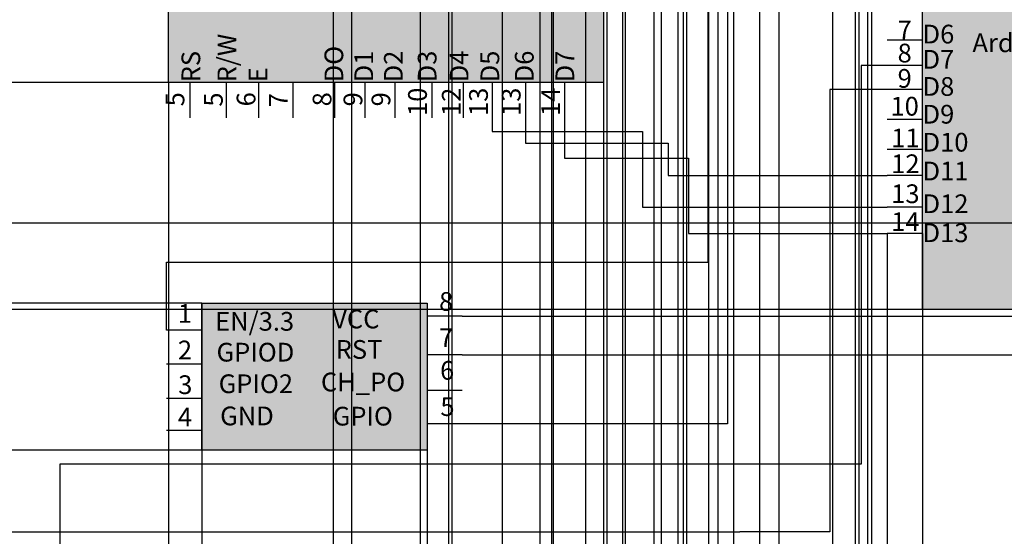
# Model space of a CAD drawing. Units: inches. Extents: x 35362 to 73946, y 43607 to 67532.
# Tile 128 of 134: x 46225 to 57838, y 50677 to 56772. Entities that reach past the tile are written whole.
import ezdxf

# ---------------------------------------------------------------- set-up
doc = ezdxf.new("R2010")
doc.units = ezdxf.units.IN
doc.header["$MEASUREMENT"] = 0
for name, color, linetype, lineweight in [('A-ANNO-DIMS', 2, 'Continuous', 18), ('E-ANNO-TEXT', 5, 'Continuous', 18), ('E-SYMB', 1, 'Continuous', 25), ('E-SYMB-PATT', 1, 'Continuous', 13), ('E-WIRE', 3, 'Continuous', 25)]:
    doc.layers.add(name, color=color, linetype=linetype, lineweight=lineweight)
doc.styles.get("Standard").update_dxf_attribs({"font": 'arial.ttf'})
doc.dimstyles.get("Standard").update_dxf_attribs({"dimtxt": 0.18, "dimasz": 0.18, "dimexe": 0.18, "dimexo": 0.0625, "dimgap": 0.09, "dimtad": 0, "dimtih": 1, "dimtoh": 1, "dimdec": 4, "dimzin": 0, "dimdsep": 46, "dimtxsty": 'Standard', "dimcen": 0.09, "dimadec": 0, "dimazin": 0, "dimtfac": 1, "dimtdec": 4, "dimtofl": 0, "dimtmove": 0, "dimatfit": 3, "dimfxl": 1, "dimtolj": 1, "dimtzin": 0, "dimarcsym": 0})

# ---------------------------------------------------------------- blocks, each defined once
blk = doc.blocks.new('*D11')
at = {"layer": 'A-ANNO-DIMS', "color": 0, "lineweight": -2, "transparency": 16777216}
for p, q in [((47979, 56029), (47979, 43607)), ((53110, 56029), (53110, 43607)), ((47979, 43607), (50544, 43607)), ((53110, 43607), (50545, 43607))]:
    blk.add_line(p, q, dxfattribs=at)
at = {"layer": 'A-ANNO-DIMS', "color": 0, "transparency": 16777216}
for points in [[(47979, 43607), (47979, 43607), (47979, 43607)], [(53110, 43607), (53110, 43607), (53110, 43607)]]:
    blk.add_solid(points, dxfattribs=at)
at = {"layer": 'Defpoints', "color": 0, "transparency": 16777216}
for p in [(47979, 56029), (53110, 56029), (53110, 43607)]:
    blk.add_point(p, dxfattribs=at)
at = {"layer": 'A-ANNO-DIMS', "color": 0, "transparency": 16777216, "insert": (50544, 43607), "char_height": 0.18, "attachment_point": 5}
blk.add_mtext('\\A1;5131', dxfattribs=at)
blk = doc.blocks.new('*D12')
at = {"layer": 'A-ANNO-DIMS', "color": 0, "lineweight": -2, "transparency": 16777216}
for p, q in [((47979, 59023), (35362, 59023)), ((35362, 59023), (35362, 57526)), ((35362, 56029), (35362, 57526)), ((47979, 56029), (35362, 56029))]:
    blk.add_line(p, q, dxfattribs=at)
at = {"layer": 'A-ANNO-DIMS', "color": 0, "transparency": 16777216}
for points in [[(35362, 59023), (35362, 59023), (35362, 59023)], [(35362, 56029), (35362, 56029), (35362, 56029)]]:
    blk.add_solid(points, dxfattribs=at)
at = {"layer": 'Defpoints', "color": 0, "transparency": 16777216}
for p in [(47979, 59023), (35362, 56029), (47979, 56029)]:
    blk.add_point(p, dxfattribs=at)
at = {"layer": 'A-ANNO-DIMS', "color": 0, "transparency": 16777216, "insert": (35362, 57526), "char_height": 0.18, "attachment_point": 5}
blk.add_mtext('\\A1;2994.4', dxfattribs=at)
blk = doc.blocks.new('*D13')
at = {"layer": 'A-ANNO-DIMS', "color": 0, "lineweight": -2, "transparency": 16777216}
for p, q in [((48373, 51694), (48373, 43607)), ((51029, 51694), (51029, 43607)), ((48374, 43607), (49701, 43607)), ((51029, 43607), (49702, 43607))]:
    blk.add_line(p, q, dxfattribs=at)
at = {"layer": 'A-ANNO-DIMS', "color": 0, "transparency": 16777216}
for points in [[(48374, 43607), (48374, 43607), (48373, 43607)], [(51029, 43607), (51029, 43607), (51029, 43607)]]:
    blk.add_solid(points, dxfattribs=at)
at = {"layer": 'Defpoints', "color": 0, "transparency": 16777216}
for p in [(48373, 51694), (51029, 51694), (51029, 43607)]:
    blk.add_point(p, dxfattribs=at)
at = {"layer": 'A-ANNO-DIMS', "color": 0, "transparency": 16777216, "insert": (49701, 43607), "char_height": 0.18, "attachment_point": 5}
blk.add_mtext('\\A1;2655.6', dxfattribs=at)
blk = doc.blocks.new('*D14')
at = {"layer": 'A-ANNO-DIMS', "color": 0, "lineweight": -2, "transparency": 16777216}
for p, q in [((48373, 53429), (35362, 53429)), ((35362, 53429), (35362, 52562)), ((35362, 51694), (35362, 52561)), ((48373, 51694), (35362, 51694))]:
    blk.add_line(p, q, dxfattribs=at)
at = {"layer": 'A-ANNO-DIMS', "color": 0, "transparency": 16777216}
for points in [[(35362, 53429), (35362, 53429), (35362, 53429)], [(35362, 51694), (35362, 51694), (35362, 51694)]]:
    blk.add_solid(points, dxfattribs=at)
at = {"layer": 'Defpoints', "color": 0, "transparency": 16777216}
for p in [(48373, 53429), (35362, 51694), (48373, 51694)]:
    blk.add_point(p, dxfattribs=at)
at = {"layer": 'A-ANNO-DIMS', "color": 0, "transparency": 16777216, "insert": (35362, 52562), "char_height": 0.18, "attachment_point": 5}
blk.add_mtext('\\A1;1735', dxfattribs=at)
blk = doc.blocks.new('*D17')
at = {"layer": 'A-ANNO-DIMS', "color": 0, "lineweight": -2, "transparency": 16777216}
for p, q in [((49923, 61293), (49923, 43607)), ((51914, 61293), (51914, 43607)), ((49923, 43607), (50918, 43607)), ((51914, 43607), (50919, 43607))]:
    blk.add_line(p, q, dxfattribs=at)
at = {"layer": 'A-ANNO-DIMS', "color": 0, "transparency": 16777216}
for points in [[(49923, 43607), (49923, 43607), (49923, 43607)], [(51914, 43607), (51914, 43607), (51914, 43607)]]:
    blk.add_solid(points, dxfattribs=at)
at = {"layer": 'Defpoints', "color": 0, "transparency": 16777216}
for p in [(49923, 61293), (51914, 61293), (51914, 43607)]:
    blk.add_point(p, dxfattribs=at)
at = {"layer": 'A-ANNO-DIMS', "color": 0, "transparency": 16777216, "insert": (50919, 43607), "char_height": 0.18, "attachment_point": 5}
blk.add_mtext('\\A1;1990.6', dxfattribs=at)
blk = doc.blocks.new('*D26')
at = {"layer": 'A-ANNO-DIMS', "color": 0, "lineweight": -2, "transparency": 16777216}
for p, q in [((47979, 56029), (35362, 56029)), ((35362, 56029), (35362, 54729)), ((35362, 53429), (35362, 54729)), ((48373, 53429), (35362, 53429))]:
    blk.add_line(p, q, dxfattribs=at)
at = {"layer": 'A-ANNO-DIMS', "color": 0, "transparency": 16777216}
for points in [[(35362, 56029), (35362, 56029), (35362, 56029)], [(35362, 53429), (35362, 53429), (35362, 53429)]]:
    blk.add_solid(points, dxfattribs=at)
at = {"layer": 'Defpoints', "color": 0, "transparency": 16777216}
for p in [(35362, 56029), (47979, 56029), (48373, 53429)]:
    blk.add_point(p, dxfattribs=at)
at = {"layer": 'A-ANNO-DIMS', "color": 0, "transparency": 16777216, "insert": (35362, 54729), "char_height": 0.18, "attachment_point": 5}
blk.add_mtext('\\A1;2599.8', dxfattribs=at)
blk = doc.blocks.new('*D27')
at = {"layer": 'A-ANNO-DIMS', "color": 0, "lineweight": -2, "transparency": 16777216}
for p, q in [((47979, 56029), (47979, 43607)), ((48373, 53429), (48373, 43607)), ((47979, 43607), (48176, 43607)), ((48373, 43607), (48176, 43607))]:
    blk.add_line(p, q, dxfattribs=at)
at = {"layer": 'A-ANNO-DIMS', "color": 0, "transparency": 16777216}
for points in [[(47979, 43607), (47979, 43607), (47979, 43607)], [(48373, 43607), (48373, 43607), (48373, 43607)]]:
    blk.add_solid(points, dxfattribs=at)
at = {"layer": 'Defpoints', "color": 0, "transparency": 16777216}
for p in [(47979, 56029), (48373, 53429), (48373, 43607)]:
    blk.add_point(p, dxfattribs=at)
at = {"layer": 'A-ANNO-DIMS', "color": 0, "transparency": 16777216, "insert": (48176, 43607), "char_height": 0.18, "attachment_point": 5}
blk.add_mtext('\\A1;394.8', dxfattribs=at)
blk = doc.blocks.new('*D36')
at = {"layer": 'A-ANNO-DIMS', "color": 0, "lineweight": -2, "transparency": 16777216}
for p, q in [((68321, 60122), (35362, 60122)), ((35362, 60122), (35362, 57248)), ((35362, 54373), (35362, 57247)), ((68321, 54373), (35362, 54373))]:
    blk.add_line(p, q, dxfattribs=at)
at = {"layer": 'A-ANNO-DIMS', "color": 0, "transparency": 16777216}
for points in [[(35362, 60122), (35362, 60122), (35362, 60122)], [(35362, 54373), (35362, 54373), (35362, 54373)]]:
    blk.add_solid(points, dxfattribs=at)
at = {"layer": 'Defpoints', "color": 0, "transparency": 16777216}
for p in [(68321, 60122), (35362, 54373), (68321, 54373)]:
    blk.add_point(p, dxfattribs=at)
at = {"layer": 'A-ANNO-DIMS', "color": 0, "transparency": 16777216, "insert": (35362, 57248), "char_height": 0.18, "attachment_point": 5}
blk.add_mtext('\\A1;5749.4', dxfattribs=at)
blk = doc.blocks.new('*D39')
at = {"layer": 'A-ANNO-DIMS', "color": 0, "lineweight": -2, "transparency": 16777216}
for p, q in [((53794, 46129), (53794, 67532)), ((53794, 67532), (54487, 67532)), ((55181, 67532), (54488, 67532)), ((55182, 46129), (55182, 67532))]:
    blk.add_line(p, q, dxfattribs=at)
at = {"layer": 'A-ANNO-DIMS', "color": 0, "transparency": 16777216}
for points in [[(53794, 67532), (53794, 67531), (53794, 67532)], [(55181, 67532), (55181, 67531), (55182, 67532)]]:
    blk.add_solid(points, dxfattribs=at)
at = {"layer": 'Defpoints', "color": 0, "transparency": 16777216}
for p in [(55182, 67532), (53794, 46129), (55182, 46129)]:
    blk.add_point(p, dxfattribs=at)
at = {"layer": 'A-ANNO-DIMS', "color": 0, "transparency": 16777216, "insert": (54488, 67532), "char_height": 0.18, "attachment_point": 5}
blk.add_mtext('\\A1;1388.0', dxfattribs=at)
blk = doc.blocks.new('*D40')
at = {"layer": 'A-ANNO-DIMS', "color": 0, "lineweight": -2, "transparency": 16777216}
for p, q in [((56874, 53352), (35362, 53352)), ((35362, 53351), (35362, 51333)), ((35362, 49315), (35362, 51333)), ((51806, 49315), (35362, 49315))]:
    blk.add_line(p, q, dxfattribs=at)
at = {"layer": 'A-ANNO-DIMS', "color": 0, "transparency": 16777216}
for points in [[(35362, 53351), (35362, 53351), (35362, 53352)], [(35362, 49315), (35362, 49315), (35362, 49315)]]:
    blk.add_solid(points, dxfattribs=at)
at = {"layer": 'Defpoints', "color": 0, "transparency": 16777216}
for p in [(35362, 53352), (56874, 53352), (51807, 49315)]:
    blk.add_point(p, dxfattribs=at)
at = {"layer": 'A-ANNO-DIMS', "color": 0, "transparency": 16777216, "insert": (35362, 51333), "char_height": 0.18, "attachment_point": 5}
blk.add_mtext('\\A1;4036.9', dxfattribs=at)
blk = doc.blocks.new('*D44')
at = {"layer": 'A-ANNO-DIMS', "color": 0, "lineweight": -2, "transparency": 16777216}
for p, q in [((52518, 64828), (52518, 43607)), ((54091, 64828), (54091, 43607)), ((52518, 43607), (53304, 43607)), ((54091, 43607), (53305, 43607))]:
    blk.add_line(p, q, dxfattribs=at)
at = {"layer": 'A-ANNO-DIMS', "color": 0, "transparency": 16777216}
for points in [[(52518, 43607), (52518, 43607), (52518, 43607)], [(54091, 43607), (54091, 43607), (54091, 43607)]]:
    blk.add_solid(points, dxfattribs=at)
at = {"layer": 'Defpoints', "color": 0, "transparency": 16777216}
for p in [(52518, 64829), (54091, 64829), (54091, 43607)]:
    blk.add_point(p, dxfattribs=at)
at = {"layer": 'A-ANNO-DIMS', "color": 0, "transparency": 16777216, "insert": (53304, 43607), "char_height": 0.18, "attachment_point": 5}
blk.add_mtext('\\A1;1573.0', dxfattribs=at)
blk = doc.blocks.new('*D49')
at = {"layer": 'A-ANNO-DIMS', "color": 0, "lineweight": -2, "transparency": 16777216}
for p, q in [((56457, 54250), (56457, 43607)), ((56874, 54250), (56874, 43607)), ((56457, 43607), (56665, 43607)), ((56873, 43607), (56666, 43607))]:
    blk.add_line(p, q, dxfattribs=at)
at = {"layer": 'A-ANNO-DIMS', "color": 0, "transparency": 16777216}
for points in [[(56457, 43607), (56457, 43607), (56457, 43607)], [(56873, 43607), (56873, 43607), (56874, 43607)]]:
    blk.add_solid(points, dxfattribs=at)
at = {"layer": 'Defpoints', "color": 0, "transparency": 16777216}
for p in [(56457, 54250), (56874, 54250), (56874, 43607)]:
    blk.add_point(p, dxfattribs=at)
at = {"layer": 'A-ANNO-DIMS', "color": 0, "transparency": 16777216, "insert": (56665, 43607), "char_height": 0.18, "attachment_point": 5}
blk.add_mtext('\\A1;416.3', dxfattribs=at)
blk = doc.blocks.new('*D53')
at = {"layer": 'A-ANNO-DIMS', "color": 0, "lineweight": -2, "transparency": 16777216}
for p, q in [((56874, 53351), (56874, 43607)), ((58225, 52935), (58225, 43607)), ((56874, 43607), (57549, 43607)), ((58225, 43607), (57550, 43607))]:
    blk.add_line(p, q, dxfattribs=at)
at = {"layer": 'A-ANNO-DIMS', "color": 0, "transparency": 16777216}
for points in [[(56874, 43607), (56874, 43607), (56874, 43607)], [(58225, 43607), (58225, 43607), (58225, 43607)]]:
    blk.add_solid(points, dxfattribs=at)
at = {"layer": 'Defpoints', "color": 0, "transparency": 16777216}
for p in [(56874, 53352), (58225, 52935), (58225, 43607)]:
    blk.add_point(p, dxfattribs=at)
at = {"layer": 'A-ANNO-DIMS', "color": 0, "transparency": 16777216, "insert": (57549, 43607), "char_height": 0.18, "attachment_point": 5}
blk.add_mtext('\\A1;1351.2', dxfattribs=at)
blk = doc.blocks.new('*D57')
at = {"layer": 'A-ANNO-DIMS', "color": 0, "lineweight": -2, "transparency": 16777216}
for p, q in [((51445, 53273), (73946, 53273)), ((73946, 53273), (73946, 53046)), ((73946, 52819), (73946, 53045)), ((51445, 52819), (73946, 52819))]:
    blk.add_line(p, q, dxfattribs=at)
at = {"layer": 'A-ANNO-DIMS', "color": 0, "transparency": 16777216}
for points in [[(73946, 53273), (73946, 53273), (73946, 53273)], [(73946, 52819), (73946, 52819), (73946, 52819)]]:
    blk.add_solid(points, dxfattribs=at)
at = {"layer": 'Defpoints', "color": 0, "transparency": 16777216}
for p in [(51445, 53273), (51445, 52819), (73946, 52819)]:
    blk.add_point(p, dxfattribs=at)
at = {"layer": 'A-ANNO-DIMS', "color": 0, "transparency": 16777216, "insert": (73946, 53046), "char_height": 0.18, "attachment_point": 5}
blk.add_mtext('\\A1;454.2', dxfattribs=at)
blk = doc.blocks.new('*D67')
at = {"layer": 'A-ANNO-DIMS', "color": 0, "lineweight": -2, "transparency": 16777216}
for p, q in [((56874, 53352), (35362, 53352)), ((35362, 53351), (35362, 49401)), ((35362, 45450), (35362, 49401)), ((53794, 45450), (35362, 45450))]:
    blk.add_line(p, q, dxfattribs=at)
at = {"layer": 'A-ANNO-DIMS', "color": 0, "transparency": 16777216}
for points in [[(35362, 53351), (35362, 53351), (35362, 53352)], [(35362, 45450), (35362, 45450), (35362, 45450)]]:
    blk.add_solid(points, dxfattribs=at)
at = {"layer": 'Defpoints', "color": 0, "transparency": 16777216}
for p in [(35362, 53352), (56874, 53352), (53794, 45450)]:
    blk.add_point(p, dxfattribs=at)
at = {"layer": 'A-ANNO-DIMS', "color": 0, "transparency": 16777216, "insert": (35362, 49401), "char_height": 0.18, "attachment_point": 5}
blk.add_mtext('\\A1;7901.6', dxfattribs=at)
blk = doc.blocks.new('*D77')
at = {"layer": 'A-ANNO-DIMS', "color": 0, "lineweight": -2, "transparency": 16777216}
for p, q in [((53794, 46129), (53794, 67532)), ((53794, 67532), (53923, 67532)), ((54053, 67532), (53924, 67532)), ((54053, 46555), (54053, 67532))]:
    blk.add_line(p, q, dxfattribs=at)
at = {"layer": 'A-ANNO-DIMS', "color": 0, "transparency": 16777216}
for points in [[(53794, 67532), (53794, 67531), (53794, 67532)], [(54053, 67532), (54053, 67531), (54053, 67532)]]:
    blk.add_solid(points, dxfattribs=at)
at = {"layer": 'Defpoints', "color": 0, "transparency": 16777216}
for p in [(54053, 67532), (54053, 46555), (53794, 46129)]:
    blk.add_point(p, dxfattribs=at)
at = {"layer": 'A-ANNO-DIMS', "color": 0, "transparency": 16777216, "insert": (53923, 67532), "char_height": 0.18, "attachment_point": 5}
blk.add_mtext('\\A1;259.26', dxfattribs=at)
blk = doc.blocks.new('*D78')
at = {"layer": 'A-ANNO-DIMS', "color": 0, "lineweight": -2, "transparency": 16777216}
for p, q in [((54053, 46555), (54053, 67532)), ((54053, 67532), (54203, 67532)), ((54353, 67532), (54203, 67532)), ((54353, 46555), (54353, 67532))]:
    blk.add_line(p, q, dxfattribs=at)
at = {"layer": 'A-ANNO-DIMS', "color": 0, "transparency": 16777216}
for points in [[(54053, 67532), (54053, 67531), (54053, 67532)], [(54353, 67532), (54353, 67531), (54353, 67532)]]:
    blk.add_solid(points, dxfattribs=at)
at = {"layer": 'Defpoints', "color": 0, "transparency": 16777216}
for p in [(54353, 67532), (54053, 46555), (54353, 46555)]:
    blk.add_point(p, dxfattribs=at)
at = {"layer": 'A-ANNO-DIMS', "color": 0, "transparency": 16777216, "insert": (54203, 67532), "char_height": 0.18, "attachment_point": 5}
blk.add_mtext('\\A1;300.2', dxfattribs=at)
blk = doc.blocks.new('*D79')
at = {"layer": 'A-ANNO-DIMS', "color": 0, "lineweight": -2, "transparency": 16777216}
for p, q in [((54353, 46555), (54353, 67532)), ((54353, 67532), (54500, 67532)), ((54648, 67532), (54501, 67532)), ((54648, 46555), (54648, 67532))]:
    blk.add_line(p, q, dxfattribs=at)
at = {"layer": 'A-ANNO-DIMS', "color": 0, "transparency": 16777216}
for points in [[(54353, 67532), (54353, 67531), (54353, 67532)], [(54648, 67532), (54648, 67531), (54648, 67532)]]:
    blk.add_solid(points, dxfattribs=at)
at = {"layer": 'Defpoints', "color": 0, "transparency": 16777216}
for p in [(54648, 67532), (54353, 46555), (54648, 46555)]:
    blk.add_point(p, dxfattribs=at)
at = {"layer": 'A-ANNO-DIMS', "color": 0, "transparency": 16777216, "insert": (54501, 67532), "char_height": 0.18, "attachment_point": 5}
blk.add_mtext('\\A1;295.1', dxfattribs=at)
blk = doc.blocks.new('*D80')
at = {"layer": 'A-ANNO-DIMS', "color": 0, "lineweight": -2, "transparency": 16777216}
for p, q in [((54648, 46555), (54648, 67532)), ((54648, 67532), (54800, 67532)), ((54953, 67532), (54801, 67532)), ((54953, 46555), (54953, 67532))]:
    blk.add_line(p, q, dxfattribs=at)
at = {"layer": 'A-ANNO-DIMS', "color": 0, "transparency": 16777216}
for points in [[(54648, 67532), (54648, 67531), (54648, 67532)], [(54953, 67532), (54953, 67531), (54953, 67532)]]:
    blk.add_solid(points, dxfattribs=at)
at = {"layer": 'Defpoints', "color": 0, "transparency": 16777216}
for p in [(54953, 67532), (54648, 46555), (54953, 46555)]:
    blk.add_point(p, dxfattribs=at)
at = {"layer": 'A-ANNO-DIMS', "color": 0, "transparency": 16777216, "insert": (54801, 67532), "char_height": 0.18, "attachment_point": 5}
blk.add_mtext('\\A1;305.27', dxfattribs=at)
blk = doc.blocks.new('*D82')
at = {"layer": 'A-ANNO-DIMS', "color": 0, "lineweight": -2, "transparency": 16777216}
for p, q in [((54464, 49315), (54464, 67532)), ((54465, 67532), (55139, 67532)), ((55815, 67532), (55140, 67532)), ((55815, 49110), (55815, 67532))]:
    blk.add_line(p, q, dxfattribs=at)
at = {"layer": 'A-ANNO-DIMS', "color": 0, "transparency": 16777216}
for points in [[(54465, 67532), (54465, 67531), (54464, 67532)], [(55815, 67532), (55815, 67531), (55815, 67532)]]:
    blk.add_solid(points, dxfattribs=at)
at = {"layer": 'Defpoints', "color": 0, "transparency": 16777216}
for p in [(55815, 67532), (54464, 49315), (55815, 49110)]:
    blk.add_point(p, dxfattribs=at)
at = {"layer": 'A-ANNO-DIMS', "color": 0, "transparency": 16777216, "insert": (55140, 67532), "char_height": 0.18, "attachment_point": 5}
blk.add_mtext('\\A1;1350.9', dxfattribs=at)
blk = doc.blocks.new('*D85')
at = {"layer": 'A-ANNO-DIMS', "color": 0, "lineweight": -2, "transparency": 16777216}
for p, q in [((50953, 49098), (50953, 67532)), ((50953, 67532), (51119, 67532)), ((51285, 67532), (51120, 67532)), ((51286, 49320), (51286, 67532))]:
    blk.add_line(p, q, dxfattribs=at)
at = {"layer": 'A-ANNO-DIMS', "color": 0, "transparency": 16777216}
for points in [[(50953, 67532), (50953, 67531), (50953, 67532)], [(51285, 67532), (51285, 67531), (51286, 67532)]]:
    blk.add_solid(points, dxfattribs=at)
at = {"layer": 'Defpoints', "color": 0, "transparency": 16777216}
for p in [(51286, 67532), (51286, 49320), (50953, 49098)]:
    blk.add_point(p, dxfattribs=at)
at = {"layer": 'A-ANNO-DIMS', "color": 0, "transparency": 16777216, "insert": (51119, 67532), "char_height": 0.18, "attachment_point": 5}
blk.add_mtext('\\A1;332.9', dxfattribs=at)
blk = doc.blocks.new('*D88')
at = {"layer": 'A-ANNO-DIMS', "color": 0, "lineweight": -2, "transparency": 16777216}
for p, q in [((52363, 48318), (52363, 67532)), ((52363, 67532), (52432, 67532)), ((52502, 67532), (52433, 67532)), ((52502, 48318), (52502, 67532))]:
    blk.add_line(p, q, dxfattribs=at)
at = {"layer": 'A-ANNO-DIMS', "color": 0, "transparency": 16777216}
for points in [[(52363, 67532), (52363, 67531), (52363, 67532)], [(52502, 67532), (52502, 67531), (52502, 67532)]]:
    blk.add_solid(points, dxfattribs=at)
at = {"layer": 'Defpoints', "color": 0, "transparency": 16777216}
for p in [(52502, 67532), (52363, 48318), (52502, 48318)]:
    blk.add_point(p, dxfattribs=at)
at = {"layer": 'A-ANNO-DIMS', "color": 0, "transparency": 16777216, "insert": (52432, 67532), "char_height": 0.18, "attachment_point": 5}
blk.add_mtext('\\A1;139.8', dxfattribs=at)
blk = doc.blocks.new('*D96')
at = {"layer": 'A-ANNO-DIMS', "color": 0, "lineweight": -2, "transparency": 16777216}
for p, q in [((53367, 64998), (53367, 43607)), ((53989, 64998), (53989, 43607)), ((53367, 43607), (53677, 43607)), ((53988, 43607), (53678, 43607))]:
    blk.add_line(p, q, dxfattribs=at)
at = {"layer": 'A-ANNO-DIMS', "color": 0, "transparency": 16777216}
for points in [[(53367, 43607), (53367, 43607), (53367, 43607)], [(53988, 43607), (53988, 43607), (53989, 43607)]]:
    blk.add_solid(points, dxfattribs=at)
at = {"layer": 'Defpoints', "color": 0, "transparency": 16777216}
for p in [(53367, 64998), (53989, 64998), (53989, 43607)]:
    blk.add_point(p, dxfattribs=at)
at = {"layer": 'A-ANNO-DIMS', "color": 0, "transparency": 16777216, "insert": (53678, 43607), "char_height": 0.18, "attachment_point": 5}
blk.add_mtext('\\A1;621.8', dxfattribs=at)
blk = doc.blocks.new('*D99')
at = {"layer": 'A-ANNO-DIMS', "color": 0, "lineweight": -2, "transparency": 16777216}
for p, q in [((52897, 65292), (52897, 43607)), ((52518, 64828), (52518, 43607)), ((52518, 43607), (52707, 43607)), ((52897, 43607), (52708, 43607))]:
    blk.add_line(p, q, dxfattribs=at)
at = {"layer": 'A-ANNO-DIMS', "color": 0, "transparency": 16777216}
for points in [[(52518, 43607), (52518, 43607), (52518, 43607)], [(52897, 43607), (52897, 43607), (52897, 43607)]]:
    blk.add_solid(points, dxfattribs=at)
at = {"layer": 'Defpoints', "color": 0, "transparency": 16777216}
for p in [(52897, 65292), (52518, 64829), (52897, 43607)]:
    blk.add_point(p, dxfattribs=at)
at = {"layer": 'A-ANNO-DIMS', "color": 0, "transparency": 16777216, "insert": (52708, 43607), "char_height": 0.18, "attachment_point": 5}
blk.add_mtext('\\A1;379.7', dxfattribs=at)
blk = doc.blocks.new('*D100')
at = {"layer": 'A-ANNO-DIMS', "color": 0, "lineweight": -2, "transparency": 16777216}
for p, q in [((52897, 65292), (52897, 43607)), ((53151, 64926), (53151, 43607)), ((52898, 43607), (53024, 43607)), ((53150, 43607), (53024, 43607))]:
    blk.add_line(p, q, dxfattribs=at)
at = {"layer": 'A-ANNO-DIMS', "color": 0, "transparency": 16777216}
for points in [[(52898, 43607), (52898, 43607), (52897, 43607)], [(53150, 43607), (53150, 43607), (53151, 43607)]]:
    blk.add_solid(points, dxfattribs=at)
at = {"layer": 'Defpoints', "color": 0, "transparency": 16777216}
for p in [(52897, 65292), (53151, 64926), (53151, 43607)]:
    blk.add_point(p, dxfattribs=at)
at = {"layer": 'A-ANNO-DIMS', "color": 0, "transparency": 16777216, "insert": (53024, 43607), "char_height": 0.18, "attachment_point": 5}
blk.add_mtext('\\A1;253.2', dxfattribs=at)
blk = doc.blocks.new('*D102')
at = {"layer": 'A-ANNO-DIMS', "color": 0, "lineweight": -2, "transparency": 16777216}
for p, q in [((56080, 63695), (56080, 43607)), ((56272, 63697), (56272, 43607)), ((56081, 43607), (56176, 43607)), ((56272, 43607), (56177, 43607))]:
    blk.add_line(p, q, dxfattribs=at)
at = {"layer": 'A-ANNO-DIMS', "color": 0, "transparency": 16777216}
for points in [[(56081, 43607), (56081, 43607), (56080, 43607)], [(56272, 43607), (56272, 43607), (56272, 43607)]]:
    blk.add_solid(points, dxfattribs=at)
at = {"layer": 'Defpoints', "color": 0, "transparency": 16777216}
for p in [(56080, 63695), (56272, 63697), (56272, 43607)]:
    blk.add_point(p, dxfattribs=at)
at = {"layer": 'A-ANNO-DIMS', "color": 0, "transparency": 16777216, "insert": (56176, 43607), "char_height": 0.18, "attachment_point": 5}
blk.add_mtext('\\A1;191.98', dxfattribs=at)
blk = doc.blocks.new('*D104')
at = {"layer": 'A-ANNO-DIMS', "color": 0, "lineweight": -2, "transparency": 16777216}
for p, q in [((56123, 63318), (56123, 43607)), ((56223, 63318), (56223, 43607)), ((56123, 43607), (56173, 43607)), ((56223, 43607), (56173, 43607))]:
    blk.add_line(p, q, dxfattribs=at)
at = {"layer": 'A-ANNO-DIMS', "color": 0, "transparency": 16777216}
for points in [[(56123, 43607), (56123, 43607), (56123, 43607)], [(56223, 43607), (56223, 43607), (56223, 43607)]]:
    blk.add_solid(points, dxfattribs=at)
at = {"layer": 'Defpoints', "color": 0, "transparency": 16777216}
for p in [(56123, 63318), (56223, 63318), (56223, 43607)]:
    blk.add_point(p, dxfattribs=at)
at = {"layer": 'A-ANNO-DIMS', "color": 0, "transparency": 16777216, "insert": (56173, 43607), "char_height": 0.18, "attachment_point": 5}
blk.add_mtext('\\A1;99.74', dxfattribs=at)
blk = doc.blocks.new('*D107')
at = {"layer": 'A-ANNO-DIMS', "color": 0, "lineweight": -2, "transparency": 16777216}
for p, q in [((50140, 59850), (50140, 43607)), ((51321, 59850), (51321, 43607)), ((50140, 43607), (50730, 43607)), ((51321, 43607), (50731, 43607))]:
    blk.add_line(p, q, dxfattribs=at)
at = {"layer": 'A-ANNO-DIMS', "color": 0, "transparency": 16777216}
for points in [[(50140, 43607), (50140, 43607), (50140, 43607)], [(51321, 43607), (51321, 43607), (51321, 43607)]]:
    blk.add_solid(points, dxfattribs=at)
at = {"layer": 'Defpoints', "color": 0, "transparency": 16777216}
for p in [(50140, 59850), (51321, 59850), (51321, 43607)]:
    blk.add_point(p, dxfattribs=at)
at = {"layer": 'A-ANNO-DIMS', "color": 0, "transparency": 16777216, "insert": (50730, 43607), "char_height": 0.18, "attachment_point": 5}
blk.add_mtext('\\A1;1181.3', dxfattribs=at)
blk = doc.blocks.new('*D112')
at = {"layer": 'A-ANNO-DIMS', "color": 0, "lineweight": -2, "transparency": 16777216}
for p, q in [((53333, 60113), (53333, 43607)), ((53705, 60126), (53705, 43607)), ((53333, 43607), (53519, 43607)), ((53705, 43607), (53519, 43607))]:
    blk.add_line(p, q, dxfattribs=at)
at = {"layer": 'A-ANNO-DIMS', "color": 0, "transparency": 16777216}
for points in [[(53333, 43607), (53333, 43607), (53333, 43607)], [(53705, 43607), (53705, 43607), (53705, 43607)]]:
    blk.add_solid(points, dxfattribs=at)
at = {"layer": 'Defpoints', "color": 0, "transparency": 16777216}
for p in [(53333, 60113), (53705, 60126), (53705, 43607)]:
    blk.add_point(p, dxfattribs=at)
at = {"layer": 'A-ANNO-DIMS', "color": 0, "transparency": 16777216, "insert": (53519, 43607), "char_height": 0.18, "attachment_point": 5}
blk.add_mtext('\\A1;372.6', dxfattribs=at)

msp = doc.modelspace()

# ---------------------------------------------------------------- hatches: boundary and pattern name
at = {"layer": 'E-SYMB-PATT'}
h = msp.add_hatch(color=256, dxfattribs=at)
h.dxf.hatch_style = 1
h.paths.add_polyline_path([(56873.602, 59185.144), (56873.602, 53351.529), (61240.907, 53351.529), (61240.907, 59185.144)])
h = msp.add_hatch(color=256, dxfattribs=at)
h.dxf.hatch_style = 1
h.paths.add_polyline_path([(53109.76, 56028.836), (53109.76, 59023.276), (47978.665, 59023.276), (47978.665, 56028.836)])
h = msp.add_hatch(color=256, dxfattribs=at)
h.dxf.hatch_style = 1
h.paths.add_polyline_path([(51029.043, 51694.087), (51029.043, 53429.019), (48373.492, 53429.019), (48373.492, 51694.087)])

# ---------------------------------------------------------------- linework, layer by layer
at = {"layer": 'E-SYMB'}
for p, q in [((56873.602, 56528.919), (56457.29, 56528.919)), ((56873.602, 56231.74), (56457.29, 56231.74)), ((48230.625, 56028.836), (48230.625, 55612.524)), ((48660.098, 56028.836), (48660.098, 55612.524)), ((49041.599, 56028.836), (49041.599, 55612.524)), ((49447.981, 56028.836), (49447.981, 55612.524)), ((49937.463, 56028.836), (49937.463, 55612.524)), ((50296.119, 56028.836), (50296.119, 55612.524)), ((50650.395, 56028.836), (50650.395, 55612.524)), ((51087.024, 56028.836), (51087.024, 55612.524)), ((51455.229, 56028.836), (51455.229, 55612.524)), ((51797.894, 56028.836), (51797.894, 55612.524)), ((52188.791, 56028.836), (52188.791, 55612.524)), ((52650.246, 56028.836), (52650.246, 55612.524)), ((56873.602, 55948.948), (56457.29, 55948.948)), ((56873.602, 55593.178), (56457.29, 55593.178)), ((56873.602, 55241.1), (56457.29, 55241.1)), ((56873.602, 54934.69), (56457.29, 54934.69)), ((56873.602, 54560.675), (56457.29, 54560.675)), ((56873.602, 54249.826), (56457.29, 54249.826)), ((51445.356, 53272.782), (51029.043, 53272.782)), ((48373.492, 53109.735), (47957.179, 53109.735)), ((51445.356, 52818.57), (51029.043, 52818.57)), ((48373.492, 52706.392), (47957.179, 52706.392)), ((51445.356, 52397.789), (51029.043, 52397.789)), ((48373.492, 52303.049), (47957.179, 52303.049)), ((48373.492, 51923.785), (47957.179, 51923.785)), ((51445.356, 52004.266), (51029.043, 52004.266))]:
    msp.add_line(p, q, dxfattribs=at)
for points in [[(56873.602, 59185.144), (61240.907, 59185.144), (61240.907, 53351.529), (56873.602, 53351.529)], [(47978.665, 59023.276), (53109.76, 59023.276), (53109.76, 56028.836), (47978.665, 56028.836)], [(48373.492, 53429.019), (51029.043, 53429.019), (51029.043, 51694.087), (48373.492, 51694.087)]]:
    msp.add_lwpolyline(points, close=True, dxfattribs=at)
at = {"layer": 'E-WIRE'}
for p, q in [((54572.84, 58474.868), (54572.84, 52004.266)), ((54344.773, 53911.892), (54344.773, 58146.959)), ((56457.29, 56231.74), (56150.086, 56231.74)), ((56150.086, 56231.74), (56150.086, 53577.957)), ((56457.29, 55948.948), (55781.317, 55948.948)), ((55781.317, 55948.948), (55781.317, 53662.393)), ((51797.894, 55612.524), (51797.894, 55453.525)), ((52188.791, 55612.524), (52188.791, 55313.853)), ((52650.246, 55612.524), (52650.246, 55136.134)), ((51797.894, 55453.525), (53572.548, 55453.525)), ((53572.548, 55453.525), (53572.548, 54560.675)), ((52188.791, 55313.853), (53871.419, 55313.853)), ((53871.419, 55313.853), (53871.419, 54934.69)), ((52650.246, 55136.134), (54114.113, 55136.134)), ((54114.113, 55136.134), (54114.113, 54249.826)), ((53871.419, 54934.69), (56457.29, 54934.69)), ((53572.548, 54560.675), (56457.29, 54560.675)), ((54114.113, 54249.826), (56457.29, 54249.826)), ((47957.179, 53109.735), (47957.179, 53911.892)), ((47957.179, 53911.892), (54344.773, 53911.892)), ((55781.317, 53662.393), (55781.317, 50729.557)), ((56150.086, 53577.957), (56150.086, 51529.852)), ((54572.84, 52004.266), (51445.356, 52004.266)), ((56150.086, 51529.852), (46698.777, 51529.852)), ((46698.777, 51529.852), (46698.777, 49689.843)), ((38575.774, 50731.821), (54718.752, 50731.821)), ((55781.317, 50729.557), (54718.752, 50731.821))]:
    msp.add_line(p, q, dxfattribs=at)

# ---------------------------------------------------------------- texts
at = {"layer": 'E-ANNO-TEXT'}
for s, height, p in [('7', 220.866, (56579.272, 56539.848)), ('D6', 220.866, (56873.602, 56491.012)), ('Arduino_UNO_R3', 220.86598, (57462.175, 56388.42)), ('8', 220.866, (56579.272, 56267.244)), ('D7', 220.866, (56873.602, 56193.637)), ('9', 220.866, (56579.272, 55968.56)), ('D8', 220.866, (56873.602, 55873.308)), ('10', 220.866, (56495.329, 55640.201)), ('D9', 220.866, (56873.602, 55545.826)), ('11', 220.866, (56504.349, 55265.371)), ('D10', 220.866, (56873.602, 55215.796)), ('12', 220.866, (56504.349, 54961.475)), ('D11', 220.866, (56873.602, 54875.374)), ('13', 220.866, (56504.349, 54607.867)), ('D12', 220.866, (56873.602, 54489.594)), ('14', 220.866, (56504.349, 54277.862)), ('D13', 220.866, (56873.602, 54147.25)), ('8', 220.866, (51171.439, 53337.11)), ('1', 220.866, (48090.611, 53195.947)), ('EN/3.3', 220.866, (48529.899, 53102.666)), ('VCC', 220.866, (49910.79, 53130.109)), ('7', 220.866, (51171.439, 52909.545)), ('2', 220.866, (48090.611, 52764.53)), ('GPIOD', 220.866, (48546.394, 52738.909)), ('RST', 220.866, (49951.348, 52771.119)), ('6', 220.866, (51183.005, 52524.352)), ('CH_PO', 220.866, (49777.527, 52386.999)), ('3', 220.866, (48094.256, 52355.135)), ('GPIO2', 220.866, (48571.252, 52366.37)), ('5', 220.866, (51186.86, 52096.787)), ('4', 220.866, (48090.401, 51973.794)), ('GND', 220.866, (48589.007, 51986.734)), ('GPIO', 220.866, (49916.584, 51983.869))]:
    msp.add_text(s, height=height, dxfattribs=at).set_placement(p)
for s, p in [('R/W', (48779.04, 56031.884)), ('DO', (50040.812, 56031.884)), ('RS ', (48353.855, 56031.884)), ('D1', (50393.227, 56031.884)), ('D2', (50742.633, 56031.884)), ('D3', (51141.004, 56031.884)), ('D4', (51518.064, 56031.884)), ('D5', (51880.508, 56031.884)), ('D6', (52286.763, 56031.884)), ('D7', (52765.285, 56031.884)), ('E ', (49144.507, 56031.884)), ('5', (48166.52, 55748.862)), ('5', (48619.301, 55745.805)), ('6', (49004.776, 55748.862)), ('7', (49386.164, 55738.929)), ('8', (49901.16, 55748.862)), ('9', (50265.572, 55748.862)), ('9', (50595.98, 55748.862)), ('10', (51027.192, 55635.623)), ('12', (51425.475, 55635.623)), ('13', (51746.704, 55635.623)), ('13', (52132.18, 55635.623)), ('14', (52597.198, 55635.623))]:
    msp.add_text(s, height=220.866, rotation=90, dxfattribs=at).set_placement(p)

# ---------------------------------------------------------------- dimensions: what is measured, and where the dimension line sits
at = {"layer": 'A-ANNO-DIMS'}
for base, p1, p2, override, picture, middle in [((51285.595, 67531.512), (50952.662, 49098.368), (51285.595, 49320.079), {"dimdec": 1, "dimlfac": 1, "dimrnd": 0, "dimzin": 0, "dimdsep": 46, "dimlunit": 2}, '*D85', (51119.128, 67531.512)), ((52502.363, 67531.512), (52362.557, 48318.269), (52502.363, 48318.269), {"dimdec": 1, "dimlfac": 1, "dimrnd": 0, "dimzin": 0, "dimdsep": 46, "dimlunit": 2}, '*D88', (52432.46, 67531.512)), ((55181.634, 67531.512), (53793.638, 46128.878), (55181.634, 46128.878), {"dimdec": 1, "dimlfac": 1, "dimrnd": 0, "dimzin": 0, "dimdsep": 46, "dimlunit": 2}, '*D39', (54487.636, 67531.512)), ((54052.899, 67531.512), (53793.638, 46128.878), (54052.899, 46555.293), {"dimdec": 2, "dimlfac": 1, "dimrnd": 0, "dimzin": 0, "dimdsep": 46, "dimlunit": 2}, '*D77', (53923.269, 67531.512)), ((54353.08, 67531.512), (54052.899, 46555.293), (54353.08, 46555.293), {"dimdec": 1, "dimlfac": 1, "dimrnd": 0, "dimzin": 0, "dimdsep": 46, "dimlunit": 2}, '*D78', (54202.99, 67531.512)), ((54648.173, 67531.512), (54353.08, 46555.293), (54648.173, 46555.293), {"dimdec": 1, "dimlfac": 1, "dimrnd": 0, "dimzin": 0, "dimdsep": 46, "dimlunit": 2}, '*D79', (54500.627, 67531.512)), ((55815.319, 67531.512), (54464.399, 49314.669), (55815.319, 49110.104), {"dimdec": 1, "dimlfac": 1, "dimrnd": 0, "dimzin": 0, "dimdsep": 46, "dimlunit": 2}, '*D82', (55139.859, 67531.512)), ((54953.441, 67531.512), (54648.173, 46555.293), (54953.441, 46555.293), {"dimdec": 2, "dimlfac": 1, "dimrnd": 0, "dimzin": 0, "dimdsep": 46, "dimlunit": 2}, '*D80', (54800.807, 67531.512)), ((52897.48, 43606.859), (52517.798, 64828.556), (52897.48, 65291.589), {"dimdec": 1, "dimlfac": 1, "dimrnd": 0, "dimzin": 0, "dimdsep": 46, "dimlunit": 2}, '*D99', (52707.639, 43606.859)), ((53150.662, 43606.859), (52897.48, 65291.589), (53150.662, 64926.138), {"dimdec": 1, "dimlfac": 1, "dimrnd": 0, "dimzin": 0, "dimdsep": 46, "dimlunit": 2}, '*D100', (53024.071, 43606.859)), ((53988.6156, 43606.859), (53366.7657, 64997.6827), (53988.6156, 64997.6827), {"dimdec": 1, "dimlfac": 1, "dimrnd": 0, "dimzin": 0, "dimdsep": 46, "dimlunit": 2}, '*D96', (53677.6907, 43606.859)), ((54090.768, 43606.859), (52517.798, 64828.556), (54090.768, 64828.556), {"dimdec": 1, "dimlfac": 1, "dimrnd": 0, "dimzin": 0, "dimdsep": 46, "dimlunit": 2}, '*D44', (53304.283, 43606.859)), ((56272.469, 43606.859), (56080.488, 63694.755), (56272.469, 63696.867), {"dimdec": 2, "dimlfac": 1, "dimrnd": 0, "dimzin": 0, "dimdsep": 46, "dimlunit": 2}, '*D102', (56176.479, 43606.859)), ((56222.953, 43606.859), (56123.213, 63318.132), (56222.953, 63318.132), {"dimdec": 2, "dimlfac": 1, "dimrnd": 0, "dimzin": 0, "dimdsep": 46, "dimlunit": 2}, '*D104', (56173.083, 43606.859)), ((51913.931, 43606.859), (49923.307, 61293.286), (51913.931, 61293.286), {"dimdec": 1, "dimlfac": 1, "dimrnd": 0, "dimzin": 0, "dimdsep": 46, "dimlunit": 2}, '*D17', (50918.619, 43606.859)), ((53705.36, 43606.859), (53332.762, 60113.464), (53705.36, 60126.3), {"dimdec": 1, "dimlfac": 1, "dimrnd": 0, "dimzin": 0, "dimdsep": 46, "dimlunit": 2}, '*D112', (53519.061, 43606.859)), ((51320.8133, 43606.859), (50139.5627, 59850.0769), (51320.8133, 59850.0769), {"dimdec": 1, "dimlfac": 1, "dimrnd": 0, "dimzin": 0, "dimdsep": 46, "dimlunit": 2}, '*D107', (50730.188, 43606.859)), ((53109.76, 43606.859), (47978.665, 56028.836), (53109.76, 56028.836), {"dimdec": 0, "dimlfac": 1, "dimrnd": 0, "dimzin": 0, "dimdsep": 46, "dimlunit": 2}, '*D11', (50544.212, 43606.859)), ((48373.492, 43606.859), (47978.665, 56028.836), (48373.492, 53429.019), {"dimdec": 1, "dimlfac": 1, "dimrnd": 0, "dimzin": 0, "dimdsep": 46, "dimlunit": 2}, '*D27', (48176.078, 43606.859)), ((56873.602, 43606.859), (56457.29, 54249.826), (56873.602, 54249.826), {"dimdec": 1, "dimlfac": 1, "dimrnd": 0, "dimzin": 0, "dimdsep": 46, "dimlunit": 2}, '*D49', (56665.446, 43606.859)), ((58224.785, 43606.859), (56873.602, 53351.529), (58224.785, 52935.216), {"dimdec": 1, "dimlfac": 1, "dimrnd": 0, "dimzin": 0, "dimdsep": 46, "dimlunit": 2}, '*D53', (57549.194, 43606.859)), ((51029.043, 43606.859), (48373.492, 51694.087), (51029.043, 51694.087), {"dimdec": 1, "dimlfac": 1, "dimrnd": 0, "dimzin": 0, "dimdsep": 46, "dimlunit": 2}, '*D13', (49701.267, 43606.859))]:
    dim = msp.add_linear_dim(base=base, p1=p1, p2=p2, dimstyle='Standard', override=override, dxfattribs=at)
    dim.commit()
    dim.dimension.update_dxf_attribs({"geometry": picture, "text_midpoint": middle})
for base, p1, p2, override, picture, middle in [((35361.949, 54372.948), (68320.871, 60122.346), (68320.871, 54372.948), {"dimdec": 1, "dimlfac": 1, "dimrnd": 0, "dimzin": 0, "dimdsep": 46, "dimlunit": 2}, '*D36', (35361.949, 57247.647)), ((35361.949, 56028.836), (47978.665, 59023.276), (47978.665, 56028.836), {"dimdec": 1, "dimlfac": 1, "dimrnd": 0, "dimzin": 0, "dimdsep": 46, "dimlunit": 2}, '*D12', (35361.949, 57526.056)), ((35361.949, 56028.836), (48373.492, 53429.019), (47978.665, 56028.836), {"dimdec": 1, "dimlfac": 1, "dimrnd": 0, "dimzin": 0, "dimdsep": 46, "dimlunit": 2}, '*D26', (35361.949, 54728.927)), ((35361.949, 51694.087), (48373.492, 53429.019), (48373.492, 51694.087), {"dimdec": 0, "dimlfac": 1, "dimrnd": 0, "dimzin": 0, "dimdsep": 46, "dimlunit": 2}, '*D14', (35361.949, 52561.553)), ((35361.949, 53351.529), (51806.517, 49314.669), (56873.602, 53351.529), {"dimdec": 1, "dimlfac": 1, "dimrnd": 0, "dimzin": 0, "dimdsep": 46, "dimlunit": 2}, '*D40', (35361.949, 51333.099)), ((35361.949, 53351.529), (53793.638, 45449.894), (56873.602, 53351.529), {"dimdec": 1, "dimlfac": 1, "dimrnd": 0, "dimzin": 0, "dimdsep": 46, "dimlunit": 2}, '*D67', (35361.949, 49400.712)), ((73945.646, 52818.57), (51445.356, 53272.782), (51445.356, 52818.57), {"dimdec": 1, "dimlfac": 1, "dimrnd": 0, "dimzin": 0, "dimdsep": 46, "dimlunit": 2}, '*D57', (73945.646, 53045.676))]:
    dim = msp.add_linear_dim(base=base, p1=p1, p2=p2, angle=90, dimstyle='Standard', override=override, dxfattribs=at)
    dim.commit()
    dim.dimension.update_dxf_attribs({"geometry": picture, "text_midpoint": middle})

doc.saveas('drawing.dxf')
